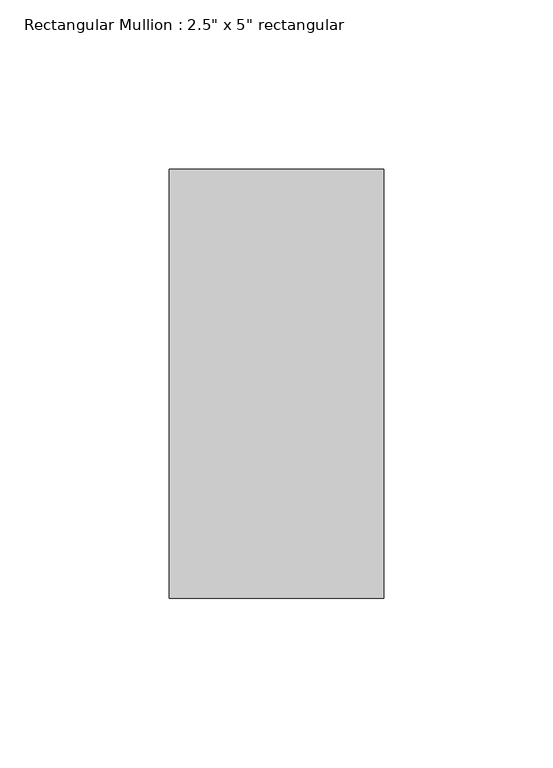
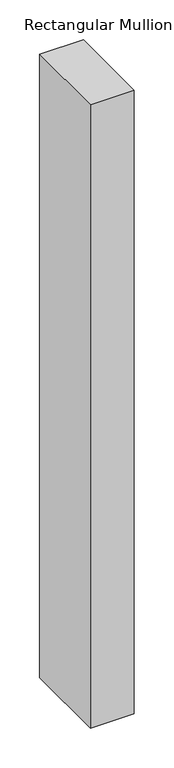
"""IFC4 building model written with IfcOpenShell, lengths in millimetres: member geometry."""

from ifc_helpers import new_model, si_unit, frame, origin, place, context, project, spatial, polyline, outline, extrude, source, transform, mapped, element, save


def member_eb96f34d(model_context):
    return source(origin(), model_context, "Body", "SweptSolid", [
        extrude(outline(polyline([(0.0, 63.5), (0.0, -63.5), (-63.5, -63.5), (-63.5, 63.5), (0.0, 63.5)])), frame((0.0, 0.0, -954.0158113), z_axis=(0.0, 0.0, 1.0), x_axis=(1.0, 0.0, 0.0)), (0.0, 0.0, 1.0), 954.0158113),
    ])


if __name__ == "__main__":
    model = new_model("IFC4")
    model_context = context("Model", 3, world=origin())
    ifc_project = project(units=[si_unit("LENGTHUNIT", "METRE", prefix="MILLI")], contexts=[model_context])
    site = spatial("IfcSite", under=ifc_project)
    building = spatial("IfcBuilding", under=site)
    placement = place(None, origin())
    member_shape = member_eb96f34d(model_context)
    element("IfcMember", 1, ObjectType="Rectangular Mullion : 2.5\" x 5\" rectangular", at=placement, inside=building, context=model_context, shape_type="MappedRepresentation", body=[
        mapped(member_shape, transform((0.0, 0.0, 0.0), x_axis=(1.0, 0.0, 0.0), y_axis=(0.0, 1.0, 0.0), z_axis=(0.0, 0.0, 1.0))),
    ])
    save(model, "model.ifc")

# Revit data of these elements
# Type "Rectangular Mullion : 2.5\" x 5\" rectangular"
#   built-in parameter 1007304 = 0.416667 (stored number, unit not read)
#   built-in parameter 1007301 = 0.104167 (stored number, unit not read)
#   built-in parameter 1007300 = 0.104167 (stored number, unit not read)
# Element 1 (IfcMember, "Rectangular Mullion : 2.5\" x 5\" rectangular")
#   Materials on its faces: "Aluminum"
# Materials
#   "Aluminum": class "Metal", colour RGB 247 247 247, transparency 0, Description = "Aluminum 6061", Cost = 0
